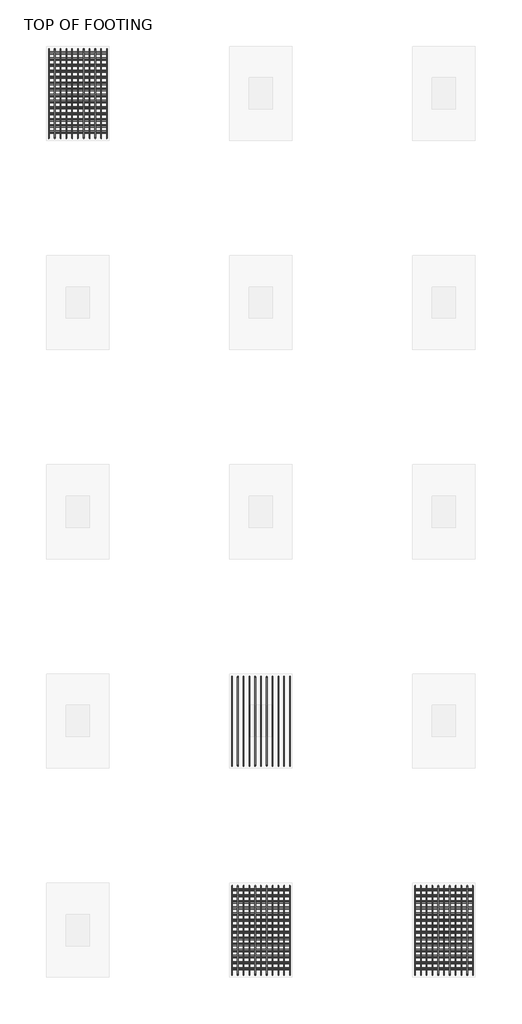
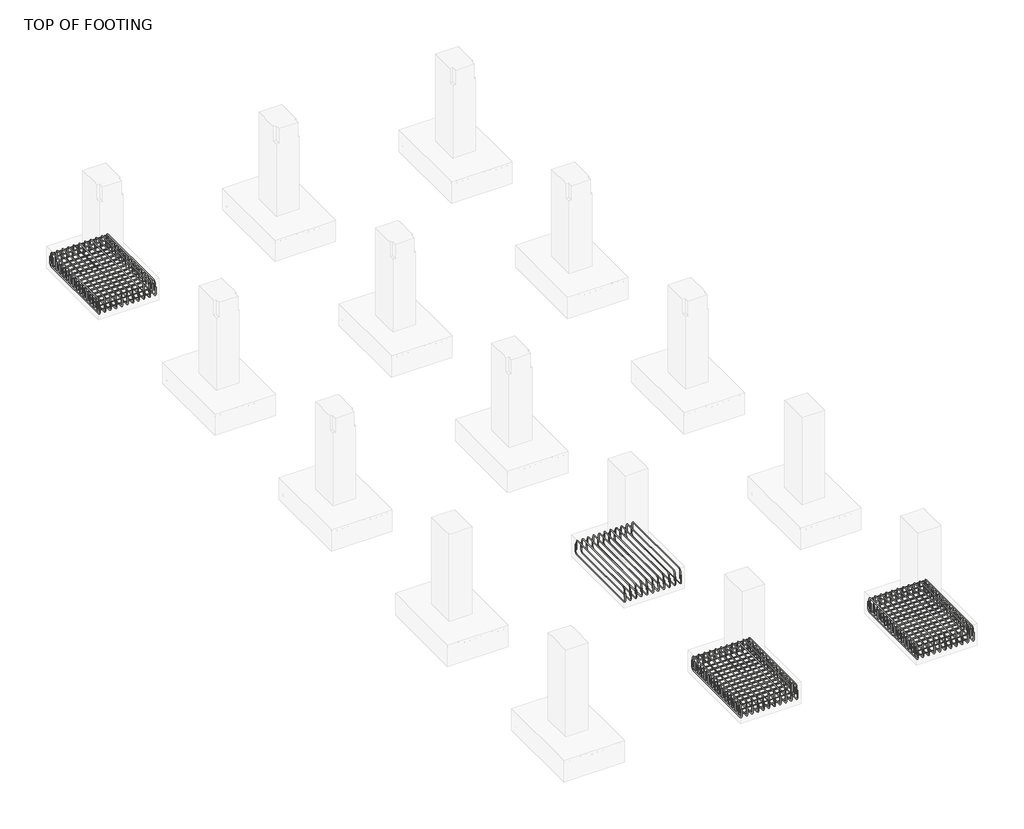
# One storey, part 7 of 11: 14 reinforcing bars.
"""IFC4 building model written with IfcOpenShell, lengths in millimetres."""

from ifc_helpers import new_model, si_unit, point, frame, origin, place, context, project, spatial, polyline, circle_curve, trimmed, segment, composite_curve, source, transform, mapped, element, save
from ifc_brep_helpers import swept_disk

model = new_model("IFC4")

# Units and contexts
model_context = context("Model", 3, world=origin())
ifc_project = project(units=[si_unit("LENGTHUNIT", "METRE", prefix="MILLI")], contexts=[model_context])

# Site, building, storey
site = spatial("IfcSite", under=ifc_project)
building = spatial("IfcBuilding", under=site)
storey = spatial("IfcBuildingStorey", under=building, Name="TOP OF FOOTING", Elevation=-1828.8)

# Reinforcing bars
placement = place(None, origin())
reinforcing_bar_shape = source(origin(), model_context, "Body", "SolidModel", [
    swept_disk(composite_curve([segment(polyline([(-1816.2384094, 18549.4712443, -2012.1658531), (-1816.2384094, 18549.4712443, -2159.4658531)]), True, "CONTINUOUS"), segment(trimmed(circle_curve(frame((-1816.2384094, 18595.8212443, -2159.4658531), z_axis=(1.0, 0.0, 0.0), x_axis=(0.0, -46.35000000000218, 0.0)), 46.35), [point((-1816.2384094, 18549.4712443, -2159.4658531))], [point((-1816.2384094, 18595.8212443, -2205.8158531))], True, "CARTESIAN"), True, "CONTINUOUS"), segment(polyline([(-1816.2384094, 18595.8212443, -2205.8158531), (-1816.2384094, 20210.4212443, -2205.8158531)]), True, "CONTINUOUS"), segment(trimmed(circle_curve(frame((-1816.2384094, 20210.4212443, -2159.4658531), z_axis=(1.0, 0.0, 0.0), x_axis=(0.0, 0.0, -46.34999999999991)), 46.35), [point((-1816.2384094, 20210.4212443, -2205.8158531))], [point((-1816.2384094, 20256.7712443, -2159.4658531))], True, "CARTESIAN"), True, "CONTINUOUS"), segment(polyline([(-1816.2384094, 20256.7712443, -2159.4658531), (-1816.2384094, 20256.7712443, -2012.1658531)]), True, "CONTINUOUS")], self_intersect=False), 6.35),
])
element("IfcReinforcingBar", 1, at=placement, inside=storey, context=model_context, shape_type="MappedRepresentation", body=[
    mapped(reinforcing_bar_shape, transform((0.0, 0.0, 0.0), x_axis=(1.0, 0.0, 0.0), y_axis=(0.0, 1.0, 0.0), z_axis=(0.0, 0.0, 1.0))),
    mapped(reinforcing_bar_shape, transform((-110.73, 0.0, 0.0), x_axis=(1.0, 0.0, 0.0), y_axis=(0.0, 1.0, 0.0), z_axis=(0.0, 0.0, 1.0))),
    mapped(reinforcing_bar_shape, transform((-221.46, 0.0, 0.0), x_axis=(1.0, 0.0, 0.0), y_axis=(0.0, 1.0, 0.0), z_axis=(0.0, 0.0, 1.0))),
    mapped(reinforcing_bar_shape, transform((-332.19, 0.0, 0.0), x_axis=(1.0, 0.0, 0.0), y_axis=(0.0, 1.0, 0.0), z_axis=(0.0, 0.0, 1.0))),
    mapped(reinforcing_bar_shape, transform((-442.92, 0.0, 0.0), x_axis=(1.0, 0.0, 0.0), y_axis=(0.0, 1.0, 0.0), z_axis=(0.0, 0.0, 1.0))),
    mapped(reinforcing_bar_shape, transform((-553.65, 0.0, 0.0), x_axis=(1.0, 0.0, 0.0), y_axis=(0.0, 1.0, 0.0), z_axis=(0.0, 0.0, 1.0))),
    mapped(reinforcing_bar_shape, transform((-664.38, 0.0, 0.0), x_axis=(1.0, 0.0, 0.0), y_axis=(0.0, 1.0, 0.0), z_axis=(0.0, 0.0, 1.0))),
    mapped(reinforcing_bar_shape, transform((-775.11, 0.0, 0.0), x_axis=(1.0, 0.0, 0.0), y_axis=(0.0, 1.0, 0.0), z_axis=(0.0, 0.0, 1.0))),
    mapped(reinforcing_bar_shape, transform((-885.84, 0.0, 0.0), x_axis=(1.0, 0.0, 0.0), y_axis=(0.0, 1.0, 0.0), z_axis=(0.0, 0.0, 1.0))),
    mapped(reinforcing_bar_shape, transform((-996.57, 0.0, 0.0), x_axis=(1.0, 0.0, 0.0), y_axis=(0.0, 1.0, 0.0), z_axis=(0.0, 0.0, 1.0))),
    mapped(reinforcing_bar_shape, transform((-1107.3, 0.0, 0.0), x_axis=(1.0, 0.0, 0.0), y_axis=(0.0, 1.0, 0.0), z_axis=(0.0, 0.0, 1.0))),
])
reinforcing_bar_2_shape = source(origin(), model_context, "Body", "SolidModel", [
    swept_disk(composite_curve([segment(polyline([(-2923.5384094, 18577.6603603, -2096.8914539), (-2923.5384094, 18577.6603603, -1949.5914539)]), True, "CONTINUOUS"), segment(trimmed(circle_curve(frame((-2923.5384094, 18624.0103603, -1949.5914539), z_axis=(-1.0, 0.0, 0.0), x_axis=(0.0, -46.349999999998545, 0.0)), 46.35), [point((-2923.5384094, 18577.6603603, -1949.5914539))], [point((-2923.5384094, 18624.0103603, -1903.2414539))], True, "CARTESIAN"), True, "CONTINUOUS"), segment(polyline([(-2923.5384094, 18624.0103603, -1903.2414539), (-2923.5384094, 20181.3238837, -1903.2414539)]), True, "CONTINUOUS"), segment(trimmed(circle_curve(frame((-2923.5384094, 20181.3238837, -1949.5914539), z_axis=(-1.0, 0.0, 0.0), x_axis=(0.0, 0.0, 46.350000000000136)), 46.35), [point((-2923.5384094, 20181.3238837, -1903.2414539))], [point((-2923.5384094, 20227.6738837, -1949.5914539))], True, "CARTESIAN"), True, "CONTINUOUS"), segment(polyline([(-2923.5384094, 20227.6738837, -1949.5914539), (-2923.5384094, 20227.6738837, -2096.8914539)]), True, "CONTINUOUS")], self_intersect=False), 6.35),
])
element("IfcReinforcingBar", 2, at=placement, inside=storey, context=model_context, shape_type="MappedRepresentation", body=[
    mapped(reinforcing_bar_2_shape, transform((0.0, 0.0, 0.0), x_axis=(1.0, 0.0, 0.0), y_axis=(0.0, 1.0, 0.0), z_axis=(0.0, 0.0, 1.0))),
    mapped(reinforcing_bar_2_shape, transform((110.73, 0.0, 0.0), x_axis=(1.0, 0.0, 0.0), y_axis=(0.0, 1.0, 0.0), z_axis=(0.0, 0.0, 1.0))),
    mapped(reinforcing_bar_2_shape, transform((221.46, 0.0, 0.0), x_axis=(1.0, 0.0, 0.0), y_axis=(0.0, 1.0, 0.0), z_axis=(0.0, 0.0, 1.0))),
    mapped(reinforcing_bar_2_shape, transform((332.19, 0.0, 0.0), x_axis=(1.0, 0.0, 0.0), y_axis=(0.0, 1.0, 0.0), z_axis=(0.0, 0.0, 1.0))),
    mapped(reinforcing_bar_2_shape, transform((442.92, 0.0, 0.0), x_axis=(1.0, 0.0, 0.0), y_axis=(0.0, 1.0, 0.0), z_axis=(0.0, 0.0, 1.0))),
    mapped(reinforcing_bar_2_shape, transform((553.65, 0.0, 0.0), x_axis=(1.0, 0.0, 0.0), y_axis=(0.0, 1.0, 0.0), z_axis=(0.0, 0.0, 1.0))),
    mapped(reinforcing_bar_2_shape, transform((664.38, 0.0, 0.0), x_axis=(1.0, 0.0, 0.0), y_axis=(0.0, 1.0, 0.0), z_axis=(0.0, 0.0, 1.0))),
    mapped(reinforcing_bar_2_shape, transform((775.11, 0.0, 0.0), x_axis=(1.0, 0.0, 0.0), y_axis=(0.0, 1.0, 0.0), z_axis=(0.0, 0.0, 1.0))),
    mapped(reinforcing_bar_2_shape, transform((885.84, 0.0, 0.0), x_axis=(1.0, 0.0, 0.0), y_axis=(0.0, 1.0, 0.0), z_axis=(0.0, 0.0, 1.0))),
    mapped(reinforcing_bar_2_shape, transform((996.57, 0.0, 0.0), x_axis=(1.0, 0.0, 0.0), y_axis=(0.0, 1.0, 0.0), z_axis=(0.0, 0.0, 1.0))),
    mapped(reinforcing_bar_2_shape, transform((1107.3, 0.0, 0.0), x_axis=(1.0, 0.0, 0.0), y_axis=(0.0, 1.0, 0.0), z_axis=(0.0, 0.0, 1.0))),
])
reinforcing_bar_3_shape = source(origin(), model_context, "Body", "SolidModel", [
    swept_disk(composite_curve([segment(polyline([(-2923.5384094, 18653.1930221, -1996.7664426), (-2923.5384094, 18653.1930221, -2144.0664426)]), True, "CONTINUOUS"), segment(trimmed(circle_curve(frame((-2877.1884094, 18653.1930221, -2144.0664426), z_axis=(0.0, -1.0, 0.0), x_axis=(-46.34999999999991, 0.0, 0.0)), 46.35), [point((-2923.5384094, 18653.1930221, -2144.0664426))], [point((-2877.1884094, 18653.1930221, -2190.4164426))], True, "CARTESIAN"), True, "CONTINUOUS"), segment(polyline([(-2877.1884094, 18653.1930221, -2190.4164426), (-1862.5884094, 18653.1930221, -2190.4164426)]), True, "CONTINUOUS"), segment(trimmed(circle_curve(frame((-1862.5884094, 18653.1930221, -2144.0664426), z_axis=(0.0, -1.0, 0.0), x_axis=(0.0, 0.0, -46.350000000000364)), 46.35), [point((-1862.5884094, 18653.1930221, -2190.4164426))], [point((-1816.2384094, 18653.1930221, -2144.0664426))], True, "CARTESIAN"), True, "CONTINUOUS"), segment(polyline([(-1816.2384094, 18653.1930221, -2144.0664426), (-1816.2384094, 18653.1930221, -1996.7664426)]), True, "CONTINUOUS")], self_intersect=False), 6.35),
])
element("IfcReinforcingBar", 3, at=placement, inside=storey, context=model_context, shape_type="MappedRepresentation", body=[
    mapped(reinforcing_bar_3_shape, transform((0.0, 0.0, 0.0), x_axis=(1.0, 0.0, 0.0), y_axis=(0.0, 1.0, 0.0), z_axis=(0.0, 0.0, 1.0))),
    mapped(reinforcing_bar_3_shape, transform((0.0, 116.2744005, 0.0), x_axis=(1.0, 0.0, 0.0), y_axis=(0.0, 1.0, 0.0), z_axis=(0.0, 0.0, 1.0))),
    mapped(reinforcing_bar_3_shape, transform((0.0, 232.5488009, 0.0), x_axis=(1.0, 0.0, 0.0), y_axis=(0.0, 1.0, 0.0), z_axis=(0.0, 0.0, 1.0))),
    mapped(reinforcing_bar_3_shape, transform((0.0, 348.8232014, 0.0), x_axis=(1.0, 0.0, 0.0), y_axis=(0.0, 1.0, 0.0), z_axis=(0.0, 0.0, 1.0))),
    mapped(reinforcing_bar_3_shape, transform((0.0, 465.0976018, 0.0), x_axis=(1.0, 0.0, 0.0), y_axis=(0.0, 1.0, 0.0), z_axis=(0.0, 0.0, 1.0))),
    mapped(reinforcing_bar_3_shape, transform((0.0, 581.3720023, 0.0), x_axis=(1.0, 0.0, 0.0), y_axis=(0.0, 1.0, 0.0), z_axis=(0.0, 0.0, 1.0))),
    mapped(reinforcing_bar_3_shape, transform((0.0, 697.6464027, 0.0), x_axis=(1.0, 0.0, 0.0), y_axis=(0.0, 1.0, 0.0), z_axis=(0.0, 0.0, 1.0))),
    mapped(reinforcing_bar_3_shape, transform((0.0, 813.9208032, 0.0), x_axis=(1.0, 0.0, 0.0), y_axis=(0.0, 1.0, 0.0), z_axis=(0.0, 0.0, 1.0))),
    mapped(reinforcing_bar_3_shape, transform((0.0, 930.1952036, 0.0), x_axis=(1.0, 0.0, 0.0), y_axis=(0.0, 1.0, 0.0), z_axis=(0.0, 0.0, 1.0))),
    mapped(reinforcing_bar_3_shape, transform((0.0, 1046.4696041, 0.0), x_axis=(1.0, 0.0, 0.0), y_axis=(0.0, 1.0, 0.0), z_axis=(0.0, 0.0, 1.0))),
    mapped(reinforcing_bar_3_shape, transform((0.0, 1162.7440045, 0.0), x_axis=(1.0, 0.0, 0.0), y_axis=(0.0, 1.0, 0.0), z_axis=(0.0, 0.0, 1.0))),
    mapped(reinforcing_bar_3_shape, transform((0.0, 1279.018405, 0.0), x_axis=(1.0, 0.0, 0.0), y_axis=(0.0, 1.0, 0.0), z_axis=(0.0, 0.0, 1.0))),
    mapped(reinforcing_bar_3_shape, transform((0.0, 1395.2928054, 0.0), x_axis=(1.0, 0.0, 0.0), y_axis=(0.0, 1.0, 0.0), z_axis=(0.0, 0.0, 1.0))),
    mapped(reinforcing_bar_3_shape, transform((0.0, 1511.5672059, 0.0), x_axis=(1.0, 0.0, 0.0), y_axis=(0.0, 1.0, 0.0), z_axis=(0.0, 0.0, 1.0))),
])
reinforcing_bar_4_shape = source(origin(), model_context, "Body", "SolidModel", [
    swept_disk(composite_curve([segment(polyline([(-2923.5384094, 20194.4257435, -2114.1958609), (-2923.5384094, 20194.4257435, -1966.8958609)]), True, "CONTINUOUS"), segment(trimmed(circle_curve(frame((-2877.1884094, 20194.4257435, -1966.8958609), z_axis=(0.0, 1.0, 0.0), x_axis=(-46.34999999999991, 0.0, 0.0)), 46.35), [point((-2923.5384094, 20194.4257435, -1966.8958609))], [point((-2877.1884094, 20194.4257435, -1920.5458609))], True, "CARTESIAN"), True, "CONTINUOUS"), segment(polyline([(-2877.1884094, 20194.4257435, -1920.5458609), (-1862.5884094, 20194.4257435, -1920.5458609)]), True, "CONTINUOUS"), segment(trimmed(circle_curve(frame((-1862.5884094, 20194.4257435, -1966.8958609), z_axis=(0.0, 1.0, 0.0), x_axis=(0.0, 0.0, 46.34999999999991)), 46.35), [point((-1862.5884094, 20194.4257435, -1920.5458609))], [point((-1816.2384094, 20194.4257435, -1966.8958609))], True, "CARTESIAN"), True, "CONTINUOUS"), segment(polyline([(-1816.2384094, 20194.4257435, -1966.8958609), (-1816.2384094, 20194.4257435, -2114.1958609)]), True, "CONTINUOUS")], self_intersect=False), 6.35),
])
element("IfcReinforcingBar", 4, at=placement, inside=storey, context=model_context, shape_type="MappedRepresentation", body=[
    mapped(reinforcing_bar_4_shape, transform((0.0, 0.0, 0.0), x_axis=(1.0, 0.0, 0.0), y_axis=(0.0, 1.0, 0.0), z_axis=(0.0, 0.0, 1.0))),
    mapped(reinforcing_bar_4_shape, transform((0.0, -116.1057918, 0.0), x_axis=(1.0, 0.0, 0.0), y_axis=(0.0, 1.0, 0.0), z_axis=(0.0, 0.0, 1.0))),
    mapped(reinforcing_bar_4_shape, transform((0.0, -232.2115836, 0.0), x_axis=(1.0, 0.0, 0.0), y_axis=(0.0, 1.0, 0.0), z_axis=(0.0, 0.0, 1.0))),
    mapped(reinforcing_bar_4_shape, transform((0.0, -348.3173754, 0.0), x_axis=(1.0, 0.0, 0.0), y_axis=(0.0, 1.0, 0.0), z_axis=(0.0, 0.0, 1.0))),
    mapped(reinforcing_bar_4_shape, transform((0.0, -464.4231672, 0.0), x_axis=(1.0, 0.0, 0.0), y_axis=(0.0, 1.0, 0.0), z_axis=(0.0, 0.0, 1.0))),
    mapped(reinforcing_bar_4_shape, transform((0.0, -580.528959, 0.0), x_axis=(1.0, 0.0, 0.0), y_axis=(0.0, 1.0, 0.0), z_axis=(0.0, 0.0, 1.0))),
    mapped(reinforcing_bar_4_shape, transform((0.0, -696.6347508, 0.0), x_axis=(1.0, 0.0, 0.0), y_axis=(0.0, 1.0, 0.0), z_axis=(0.0, 0.0, 1.0))),
    mapped(reinforcing_bar_4_shape, transform((0.0, -812.7405426, 0.0), x_axis=(1.0, 0.0, 0.0), y_axis=(0.0, 1.0, 0.0), z_axis=(0.0, 0.0, 1.0))),
    mapped(reinforcing_bar_4_shape, transform((0.0, -928.8463344, 0.0), x_axis=(1.0, 0.0, 0.0), y_axis=(0.0, 1.0, 0.0), z_axis=(0.0, 0.0, 1.0))),
    mapped(reinforcing_bar_4_shape, transform((0.0, -1044.9521262, 0.0), x_axis=(1.0, 0.0, 0.0), y_axis=(0.0, 1.0, 0.0), z_axis=(0.0, 0.0, 1.0))),
    mapped(reinforcing_bar_4_shape, transform((0.0, -1161.057918, 0.0), x_axis=(1.0, 0.0, 0.0), y_axis=(0.0, 1.0, 0.0), z_axis=(0.0, 0.0, 1.0))),
    mapped(reinforcing_bar_4_shape, transform((0.0, -1277.1637098, 0.0), x_axis=(1.0, 0.0, 0.0), y_axis=(0.0, 1.0, 0.0), z_axis=(0.0, 0.0, 1.0))),
    mapped(reinforcing_bar_4_shape, transform((0.0, -1393.2695016, 0.0), x_axis=(1.0, 0.0, 0.0), y_axis=(0.0, 1.0, 0.0), z_axis=(0.0, 0.0, 1.0))),
    mapped(reinforcing_bar_4_shape, transform((0.0, -1509.3752934, 0.0), x_axis=(1.0, 0.0, 0.0), y_axis=(0.0, 1.0, 0.0), z_axis=(0.0, 0.0, 1.0))),
])
reinforcing_bar_5_shape = source(origin(), model_context, "Body", "SolidModel", [
    swept_disk(composite_curve([segment(polyline([(5183.7615906, 2549.4712443, -2012.1658531), (5183.7615906, 2549.4712443, -2159.4658531)]), True, "CONTINUOUS"), segment(trimmed(circle_curve(frame((5183.7615906, 2595.8212443, -2159.4658531), z_axis=(1.0, 0.0, 0.0), x_axis=(0.0, -46.350000000000364, 0.0)), 46.35), [point((5183.7615906, 2549.4712443, -2159.4658531))], [point((5183.7615906, 2595.8212443, -2205.8158531))], True, "CARTESIAN"), True, "CONTINUOUS"), segment(polyline([(5183.7615906, 2595.8212443, -2205.8158531), (5183.7615906, 4210.4212443, -2205.8158531)]), True, "CONTINUOUS"), segment(trimmed(circle_curve(frame((5183.7615906, 4210.4212443, -2159.4658531), z_axis=(1.0, 0.0, 0.0), x_axis=(0.0, 0.0, -46.34999999999991)), 46.35), [point((5183.7615906, 4210.4212443, -2205.8158531))], [point((5183.7615906, 4256.7712443, -2159.4658531))], True, "CARTESIAN"), True, "CONTINUOUS"), segment(polyline([(5183.7615906, 4256.7712443, -2159.4658531), (5183.7615906, 4256.7712443, -2012.1658531)]), True, "CONTINUOUS")], self_intersect=False), 6.35),
])
element("IfcReinforcingBar", 5, at=placement, inside=storey, context=model_context, shape_type="MappedRepresentation", body=[
    mapped(reinforcing_bar_5_shape, transform((0.0, 0.0, 0.0), x_axis=(1.0, 0.0, 0.0), y_axis=(0.0, 1.0, 0.0), z_axis=(0.0, 0.0, 1.0))),
    mapped(reinforcing_bar_5_shape, transform((-110.73, 0.0, 0.0), x_axis=(1.0, 0.0, 0.0), y_axis=(0.0, 1.0, 0.0), z_axis=(0.0, 0.0, 1.0))),
    mapped(reinforcing_bar_5_shape, transform((-221.46, 0.0, 0.0), x_axis=(1.0, 0.0, 0.0), y_axis=(0.0, 1.0, 0.0), z_axis=(0.0, 0.0, 1.0))),
    mapped(reinforcing_bar_5_shape, transform((-332.19, 0.0, 0.0), x_axis=(1.0, 0.0, 0.0), y_axis=(0.0, 1.0, 0.0), z_axis=(0.0, 0.0, 1.0))),
    mapped(reinforcing_bar_5_shape, transform((-442.92, 0.0, 0.0), x_axis=(1.0, 0.0, 0.0), y_axis=(0.0, 1.0, 0.0), z_axis=(0.0, 0.0, 1.0))),
    mapped(reinforcing_bar_5_shape, transform((-553.65, 0.0, 0.0), x_axis=(1.0, 0.0, 0.0), y_axis=(0.0, 1.0, 0.0), z_axis=(0.0, 0.0, 1.0))),
    mapped(reinforcing_bar_5_shape, transform((-664.38, 0.0, 0.0), x_axis=(1.0, 0.0, 0.0), y_axis=(0.0, 1.0, 0.0), z_axis=(0.0, 0.0, 1.0))),
    mapped(reinforcing_bar_5_shape, transform((-775.11, 0.0, 0.0), x_axis=(1.0, 0.0, 0.0), y_axis=(0.0, 1.0, 0.0), z_axis=(0.0, 0.0, 1.0))),
    mapped(reinforcing_bar_5_shape, transform((-885.84, 0.0, 0.0), x_axis=(1.0, 0.0, 0.0), y_axis=(0.0, 1.0, 0.0), z_axis=(0.0, 0.0, 1.0))),
    mapped(reinforcing_bar_5_shape, transform((-996.57, 0.0, 0.0), x_axis=(1.0, 0.0, 0.0), y_axis=(0.0, 1.0, 0.0), z_axis=(0.0, 0.0, 1.0))),
    mapped(reinforcing_bar_5_shape, transform((-1107.3, 0.0, 0.0), x_axis=(1.0, 0.0, 0.0), y_axis=(0.0, 1.0, 0.0), z_axis=(0.0, 0.0, 1.0))),
])
reinforcing_bar_6_shape = source(origin(), model_context, "Body", "SolidModel", [
    swept_disk(composite_curve([segment(polyline([(4076.4615906, 2577.6603603, -2096.8914539), (4076.4615906, 2577.6603603, -1949.5914539)]), True, "CONTINUOUS"), segment(trimmed(circle_curve(frame((4076.4615906, 2624.0103603, -1949.5914539), z_axis=(-1.0, 0.0, 0.0), x_axis=(0.0, -46.34999999999991, 0.0)), 46.35), [point((4076.4615906, 2577.6603603, -1949.5914539))], [point((4076.4615906, 2624.0103603, -1903.2414539))], True, "CARTESIAN"), True, "CONTINUOUS"), segment(polyline([(4076.4615906, 2624.0103603, -1903.2414539), (4076.4615906, 4181.3238837, -1903.2414539)]), True, "CONTINUOUS"), segment(trimmed(circle_curve(frame((4076.4615906, 4181.3238837, -1949.5914539), z_axis=(-1.0, 0.0, 0.0), x_axis=(0.0, 0.0, 46.350000000000136)), 46.35), [point((4076.4615906, 4181.3238837, -1903.2414539))], [point((4076.4615906, 4227.6738837, -1949.5914539))], True, "CARTESIAN"), True, "CONTINUOUS"), segment(polyline([(4076.4615906, 4227.6738837, -1949.5914539), (4076.4615906, 4227.6738837, -2096.8914539)]), True, "CONTINUOUS")], self_intersect=False), 6.35),
])
element("IfcReinforcingBar", 6, at=placement, inside=storey, context=model_context, shape_type="MappedRepresentation", body=[
    mapped(reinforcing_bar_6_shape, transform((0.0, 0.0, 0.0), x_axis=(1.0, 0.0, 0.0), y_axis=(0.0, 1.0, 0.0), z_axis=(0.0, 0.0, 1.0))),
    mapped(reinforcing_bar_6_shape, transform((110.73, 0.0, 0.0), x_axis=(1.0, 0.0, 0.0), y_axis=(0.0, 1.0, 0.0), z_axis=(0.0, 0.0, 1.0))),
    mapped(reinforcing_bar_6_shape, transform((221.46, 0.0, 0.0), x_axis=(1.0, 0.0, 0.0), y_axis=(0.0, 1.0, 0.0), z_axis=(0.0, 0.0, 1.0))),
    mapped(reinforcing_bar_6_shape, transform((332.19, 0.0, 0.0), x_axis=(1.0, 0.0, 0.0), y_axis=(0.0, 1.0, 0.0), z_axis=(0.0, 0.0, 1.0))),
    mapped(reinforcing_bar_6_shape, transform((442.92, 0.0, 0.0), x_axis=(1.0, 0.0, 0.0), y_axis=(0.0, 1.0, 0.0), z_axis=(0.0, 0.0, 1.0))),
    mapped(reinforcing_bar_6_shape, transform((553.65, 0.0, 0.0), x_axis=(1.0, 0.0, 0.0), y_axis=(0.0, 1.0, 0.0), z_axis=(0.0, 0.0, 1.0))),
    mapped(reinforcing_bar_6_shape, transform((664.38, 0.0, 0.0), x_axis=(1.0, 0.0, 0.0), y_axis=(0.0, 1.0, 0.0), z_axis=(0.0, 0.0, 1.0))),
    mapped(reinforcing_bar_6_shape, transform((775.11, 0.0, 0.0), x_axis=(1.0, 0.0, 0.0), y_axis=(0.0, 1.0, 0.0), z_axis=(0.0, 0.0, 1.0))),
    mapped(reinforcing_bar_6_shape, transform((885.84, 0.0, 0.0), x_axis=(1.0, 0.0, 0.0), y_axis=(0.0, 1.0, 0.0), z_axis=(0.0, 0.0, 1.0))),
    mapped(reinforcing_bar_6_shape, transform((996.57, 0.0, 0.0), x_axis=(1.0, 0.0, 0.0), y_axis=(0.0, 1.0, 0.0), z_axis=(0.0, 0.0, 1.0))),
    mapped(reinforcing_bar_6_shape, transform((1107.3, 0.0, 0.0), x_axis=(1.0, 0.0, 0.0), y_axis=(0.0, 1.0, 0.0), z_axis=(0.0, 0.0, 1.0))),
])
reinforcing_bar_7_shape = source(origin(), model_context, "Body", "SolidModel", [
    swept_disk(composite_curve([segment(polyline([(4076.4615906, 2653.1930221, -1996.7664426), (4076.4615906, 2653.1930221, -2144.0664426)]), True, "CONTINUOUS"), segment(trimmed(circle_curve(frame((4122.8115906, 2653.1930221, -2144.0664426), z_axis=(0.0, -1.0, 0.0), x_axis=(-46.350000000000364, 0.0, 0.0)), 46.35), [point((4076.4615906, 2653.1930221, -2144.0664426))], [point((4122.8115906, 2653.1930221, -2190.4164426))], True, "CARTESIAN"), True, "CONTINUOUS"), segment(polyline([(4122.8115906, 2653.1930221, -2190.4164426), (5137.4115906, 2653.1930221, -2190.4164426)]), True, "CONTINUOUS"), segment(trimmed(circle_curve(frame((5137.4115906, 2653.1930221, -2144.0664426), z_axis=(0.0, -1.0, 0.0), x_axis=(0.0, 0.0, -46.350000000000364)), 46.35), [point((5137.4115906, 2653.1930221, -2190.4164426))], [point((5183.7615906, 2653.1930221, -2144.0664426))], True, "CARTESIAN"), True, "CONTINUOUS"), segment(polyline([(5183.7615906, 2653.1930221, -2144.0664426), (5183.7615906, 2653.1930221, -1996.7664426)]), True, "CONTINUOUS")], self_intersect=False), 6.35),
])
element("IfcReinforcingBar", 7, at=placement, inside=storey, context=model_context, shape_type="MappedRepresentation", body=[
    mapped(reinforcing_bar_7_shape, transform((0.0, 0.0, 0.0), x_axis=(1.0, 0.0, 0.0), y_axis=(0.0, 1.0, 0.0), z_axis=(0.0, 0.0, 1.0))),
    mapped(reinforcing_bar_7_shape, transform((0.0, 116.2744005, 0.0), x_axis=(1.0, 0.0, 0.0), y_axis=(0.0, 1.0, 0.0), z_axis=(0.0, 0.0, 1.0))),
    mapped(reinforcing_bar_7_shape, transform((0.0, 232.5488009, 0.0), x_axis=(1.0, 0.0, 0.0), y_axis=(0.0, 1.0, 0.0), z_axis=(0.0, 0.0, 1.0))),
    mapped(reinforcing_bar_7_shape, transform((0.0, 348.8232014, 0.0), x_axis=(1.0, 0.0, 0.0), y_axis=(0.0, 1.0, 0.0), z_axis=(0.0, 0.0, 1.0))),
    mapped(reinforcing_bar_7_shape, transform((0.0, 465.0976018, 0.0), x_axis=(1.0, 0.0, 0.0), y_axis=(0.0, 1.0, 0.0), z_axis=(0.0, 0.0, 1.0))),
    mapped(reinforcing_bar_7_shape, transform((0.0, 581.3720023, 0.0), x_axis=(1.0, 0.0, 0.0), y_axis=(0.0, 1.0, 0.0), z_axis=(0.0, 0.0, 1.0))),
    mapped(reinforcing_bar_7_shape, transform((0.0, 697.6464027, 0.0), x_axis=(1.0, 0.0, 0.0), y_axis=(0.0, 1.0, 0.0), z_axis=(0.0, 0.0, 1.0))),
    mapped(reinforcing_bar_7_shape, transform((0.0, 813.9208032, 0.0), x_axis=(1.0, 0.0, 0.0), y_axis=(0.0, 1.0, 0.0), z_axis=(0.0, 0.0, 1.0))),
    mapped(reinforcing_bar_7_shape, transform((0.0, 930.1952036, 0.0), x_axis=(1.0, 0.0, 0.0), y_axis=(0.0, 1.0, 0.0), z_axis=(0.0, 0.0, 1.0))),
    mapped(reinforcing_bar_7_shape, transform((0.0, 1046.4696041, 0.0), x_axis=(1.0, 0.0, 0.0), y_axis=(0.0, 1.0, 0.0), z_axis=(0.0, 0.0, 1.0))),
    mapped(reinforcing_bar_7_shape, transform((0.0, 1162.7440045, 0.0), x_axis=(1.0, 0.0, 0.0), y_axis=(0.0, 1.0, 0.0), z_axis=(0.0, 0.0, 1.0))),
    mapped(reinforcing_bar_7_shape, transform((0.0, 1279.018405, 0.0), x_axis=(1.0, 0.0, 0.0), y_axis=(0.0, 1.0, 0.0), z_axis=(0.0, 0.0, 1.0))),
    mapped(reinforcing_bar_7_shape, transform((0.0, 1395.2928054, 0.0), x_axis=(1.0, 0.0, 0.0), y_axis=(0.0, 1.0, 0.0), z_axis=(0.0, 0.0, 1.0))),
    mapped(reinforcing_bar_7_shape, transform((0.0, 1511.5672059, 0.0), x_axis=(1.0, 0.0, 0.0), y_axis=(0.0, 1.0, 0.0), z_axis=(0.0, 0.0, 1.0))),
])
reinforcing_bar_8_shape = source(origin(), model_context, "Body", "SolidModel", [
    swept_disk(composite_curve([segment(polyline([(4076.4615906, 4194.4257435, -2114.1958609), (4076.4615906, 4194.4257435, -1966.8958609)]), True, "CONTINUOUS"), segment(trimmed(circle_curve(frame((4122.8115906, 4194.4257435, -1966.8958609), z_axis=(0.0, 1.0, 0.0), x_axis=(-46.350000000000364, 0.0, 0.0)), 46.35), [point((4076.4615906, 4194.4257435, -1966.8958609))], [point((4122.8115906, 4194.4257435, -1920.5458609))], True, "CARTESIAN"), True, "CONTINUOUS"), segment(polyline([(4122.8115906, 4194.4257435, -1920.5458609), (5137.4115906, 4194.4257435, -1920.5458609)]), True, "CONTINUOUS"), segment(trimmed(circle_curve(frame((5137.4115906, 4194.4257435, -1966.8958609), z_axis=(0.0, 1.0, 0.0), x_axis=(0.0, 0.0, 46.34999999999991)), 46.35), [point((5137.4115906, 4194.4257435, -1920.5458609))], [point((5183.7615906, 4194.4257435, -1966.8958609))], True, "CARTESIAN"), True, "CONTINUOUS"), segment(polyline([(5183.7615906, 4194.4257435, -1966.8958609), (5183.7615906, 4194.4257435, -2114.1958609)]), True, "CONTINUOUS")], self_intersect=False), 6.35),
])
element("IfcReinforcingBar", 8, at=placement, inside=storey, context=model_context, shape_type="MappedRepresentation", body=[
    mapped(reinforcing_bar_8_shape, transform((0.0, 0.0, 0.0), x_axis=(1.0, 0.0, 0.0), y_axis=(0.0, 1.0, 0.0), z_axis=(0.0, 0.0, 1.0))),
    mapped(reinforcing_bar_8_shape, transform((0.0, -116.1057918, 0.0), x_axis=(1.0, 0.0, 0.0), y_axis=(0.0, 1.0, 0.0), z_axis=(0.0, 0.0, 1.0))),
    mapped(reinforcing_bar_8_shape, transform((0.0, -232.2115836, 0.0), x_axis=(1.0, 0.0, 0.0), y_axis=(0.0, 1.0, 0.0), z_axis=(0.0, 0.0, 1.0))),
    mapped(reinforcing_bar_8_shape, transform((0.0, -348.3173754, 0.0), x_axis=(1.0, 0.0, 0.0), y_axis=(0.0, 1.0, 0.0), z_axis=(0.0, 0.0, 1.0))),
    mapped(reinforcing_bar_8_shape, transform((0.0, -464.4231672, 0.0), x_axis=(1.0, 0.0, 0.0), y_axis=(0.0, 1.0, 0.0), z_axis=(0.0, 0.0, 1.0))),
    mapped(reinforcing_bar_8_shape, transform((0.0, -580.528959, 0.0), x_axis=(1.0, 0.0, 0.0), y_axis=(0.0, 1.0, 0.0), z_axis=(0.0, 0.0, 1.0))),
    mapped(reinforcing_bar_8_shape, transform((0.0, -696.6347508, 0.0), x_axis=(1.0, 0.0, 0.0), y_axis=(0.0, 1.0, 0.0), z_axis=(0.0, 0.0, 1.0))),
    mapped(reinforcing_bar_8_shape, transform((0.0, -812.7405426, 0.0), x_axis=(1.0, 0.0, 0.0), y_axis=(0.0, 1.0, 0.0), z_axis=(0.0, 0.0, 1.0))),
    mapped(reinforcing_bar_8_shape, transform((0.0, -928.8463344, 0.0), x_axis=(1.0, 0.0, 0.0), y_axis=(0.0, 1.0, 0.0), z_axis=(0.0, 0.0, 1.0))),
    mapped(reinforcing_bar_8_shape, transform((0.0, -1044.9521262, 0.0), x_axis=(1.0, 0.0, 0.0), y_axis=(0.0, 1.0, 0.0), z_axis=(0.0, 0.0, 1.0))),
    mapped(reinforcing_bar_8_shape, transform((0.0, -1161.057918, 0.0), x_axis=(1.0, 0.0, 0.0), y_axis=(0.0, 1.0, 0.0), z_axis=(0.0, 0.0, 1.0))),
    mapped(reinforcing_bar_8_shape, transform((0.0, -1277.1637098, 0.0), x_axis=(1.0, 0.0, 0.0), y_axis=(0.0, 1.0, 0.0), z_axis=(0.0, 0.0, 1.0))),
    mapped(reinforcing_bar_8_shape, transform((0.0, -1393.2695016, 0.0), x_axis=(1.0, 0.0, 0.0), y_axis=(0.0, 1.0, 0.0), z_axis=(0.0, 0.0, 1.0))),
    mapped(reinforcing_bar_8_shape, transform((0.0, -1509.3752934, 0.0), x_axis=(1.0, 0.0, 0.0), y_axis=(0.0, 1.0, 0.0), z_axis=(0.0, 0.0, 1.0))),
])
reinforcing_bar_9_shape = source(origin(), model_context, "Body", "SolidModel", [
    swept_disk(composite_curve([segment(polyline([(1683.7615906, 6549.4712443, -2012.1658531), (1683.7615906, 6549.4712443, -2159.4658531)]), True, "CONTINUOUS"), segment(trimmed(circle_curve(frame((1683.7615906, 6595.8212443, -2159.4658531), z_axis=(1.0, 0.0, 0.0), x_axis=(0.0, -46.350000000000364, 0.0)), 46.35), [point((1683.7615906, 6549.4712443, -2159.4658531))], [point((1683.7615906, 6595.8212443, -2205.8158531))], True, "CARTESIAN"), True, "CONTINUOUS"), segment(polyline([(1683.7615906, 6595.8212443, -2205.8158531), (1683.7615906, 8210.4212443, -2205.8158531)]), True, "CONTINUOUS"), segment(trimmed(circle_curve(frame((1683.7615906, 8210.4212443, -2159.4658531), z_axis=(1.0, 0.0, 0.0), x_axis=(0.0, 0.0, -46.34999999999991)), 46.35), [point((1683.7615906, 8210.4212443, -2205.8158531))], [point((1683.7615906, 8256.7712443, -2159.4658531))], True, "CARTESIAN"), True, "CONTINUOUS"), segment(polyline([(1683.7615906, 8256.7712443, -2159.4658531), (1683.7615906, 8256.7712443, -2012.1658531)]), True, "CONTINUOUS")], self_intersect=False), 6.35),
])
element("IfcReinforcingBar", 9, at=placement, inside=storey, context=model_context, shape_type="MappedRepresentation", body=[
    mapped(reinforcing_bar_9_shape, transform((0.0, 0.0, 0.0), x_axis=(1.0, 0.0, 0.0), y_axis=(0.0, 1.0, 0.0), z_axis=(0.0, 0.0, 1.0))),
    mapped(reinforcing_bar_9_shape, transform((-110.73, 0.0, 0.0), x_axis=(1.0, 0.0, 0.0), y_axis=(0.0, 1.0, 0.0), z_axis=(0.0, 0.0, 1.0))),
    mapped(reinforcing_bar_9_shape, transform((-221.46, 0.0, 0.0), x_axis=(1.0, 0.0, 0.0), y_axis=(0.0, 1.0, 0.0), z_axis=(0.0, 0.0, 1.0))),
    mapped(reinforcing_bar_9_shape, transform((-332.19, 0.0, 0.0), x_axis=(1.0, 0.0, 0.0), y_axis=(0.0, 1.0, 0.0), z_axis=(0.0, 0.0, 1.0))),
    mapped(reinforcing_bar_9_shape, transform((-442.92, 0.0, 0.0), x_axis=(1.0, 0.0, 0.0), y_axis=(0.0, 1.0, 0.0), z_axis=(0.0, 0.0, 1.0))),
    mapped(reinforcing_bar_9_shape, transform((-553.65, 0.0, 0.0), x_axis=(1.0, 0.0, 0.0), y_axis=(0.0, 1.0, 0.0), z_axis=(0.0, 0.0, 1.0))),
    mapped(reinforcing_bar_9_shape, transform((-664.38, 0.0, 0.0), x_axis=(1.0, 0.0, 0.0), y_axis=(0.0, 1.0, 0.0), z_axis=(0.0, 0.0, 1.0))),
    mapped(reinforcing_bar_9_shape, transform((-775.11, 0.0, 0.0), x_axis=(1.0, 0.0, 0.0), y_axis=(0.0, 1.0, 0.0), z_axis=(0.0, 0.0, 1.0))),
    mapped(reinforcing_bar_9_shape, transform((-885.84, 0.0, 0.0), x_axis=(1.0, 0.0, 0.0), y_axis=(0.0, 1.0, 0.0), z_axis=(0.0, 0.0, 1.0))),
    mapped(reinforcing_bar_9_shape, transform((-996.57, 0.0, 0.0), x_axis=(1.0, 0.0, 0.0), y_axis=(0.0, 1.0, 0.0), z_axis=(0.0, 0.0, 1.0))),
    mapped(reinforcing_bar_9_shape, transform((-1107.3, 0.0, 0.0), x_axis=(1.0, 0.0, 0.0), y_axis=(0.0, 1.0, 0.0), z_axis=(0.0, 0.0, 1.0))),
])
reinforcing_bar_10_shape = source(origin(), model_context, "Body", "SolidModel", [
    swept_disk(composite_curve([segment(polyline([(576.4615906, 6577.6603603, -2096.8914539), (576.4615906, 6577.6603603, -1949.5914539)]), True, "CONTINUOUS"), segment(trimmed(circle_curve(frame((576.4615906, 6624.0103603, -1949.5914539), z_axis=(-1.0, 0.0, 0.0), x_axis=(0.0, -46.349999999999454, 0.0)), 46.35), [point((576.4615906, 6577.6603603, -1949.5914539))], [point((576.4615906, 6624.0103603, -1903.2414539))], True, "CARTESIAN"), True, "CONTINUOUS"), segment(polyline([(576.4615906, 6624.0103603, -1903.2414539), (576.4615906, 8181.3238837, -1903.2414539)]), True, "CONTINUOUS"), segment(trimmed(circle_curve(frame((576.4615906, 8181.3238837, -1949.5914539), z_axis=(-1.0, 0.0, 0.0), x_axis=(0.0, 0.0, 46.350000000000136)), 46.35), [point((576.4615906, 8181.3238837, -1903.2414539))], [point((576.4615906, 8227.6738837, -1949.5914539))], True, "CARTESIAN"), True, "CONTINUOUS"), segment(polyline([(576.4615906, 8227.6738837, -1949.5914539), (576.4615906, 8227.6738837, -2096.8914539)]), True, "CONTINUOUS")], self_intersect=False), 6.35),
])
element("IfcReinforcingBar", 10, at=placement, inside=storey, context=model_context, shape_type="MappedRepresentation", body=[
    mapped(reinforcing_bar_10_shape, transform((0.0, 0.0, 0.0), x_axis=(1.0, 0.0, 0.0), y_axis=(0.0, 1.0, 0.0), z_axis=(0.0, 0.0, 1.0))),
    mapped(reinforcing_bar_10_shape, transform((110.73, 0.0, 0.0), x_axis=(1.0, 0.0, 0.0), y_axis=(0.0, 1.0, 0.0), z_axis=(0.0, 0.0, 1.0))),
    mapped(reinforcing_bar_10_shape, transform((221.46, 0.0, 0.0), x_axis=(1.0, 0.0, 0.0), y_axis=(0.0, 1.0, 0.0), z_axis=(0.0, 0.0, 1.0))),
    mapped(reinforcing_bar_10_shape, transform((332.19, 0.0, 0.0), x_axis=(1.0, 0.0, 0.0), y_axis=(0.0, 1.0, 0.0), z_axis=(0.0, 0.0, 1.0))),
    mapped(reinforcing_bar_10_shape, transform((442.92, 0.0, 0.0), x_axis=(1.0, 0.0, 0.0), y_axis=(0.0, 1.0, 0.0), z_axis=(0.0, 0.0, 1.0))),
    mapped(reinforcing_bar_10_shape, transform((553.65, 0.0, 0.0), x_axis=(1.0, 0.0, 0.0), y_axis=(0.0, 1.0, 0.0), z_axis=(0.0, 0.0, 1.0))),
    mapped(reinforcing_bar_10_shape, transform((664.38, 0.0, 0.0), x_axis=(1.0, 0.0, 0.0), y_axis=(0.0, 1.0, 0.0), z_axis=(0.0, 0.0, 1.0))),
    mapped(reinforcing_bar_10_shape, transform((775.11, 0.0, 0.0), x_axis=(1.0, 0.0, 0.0), y_axis=(0.0, 1.0, 0.0), z_axis=(0.0, 0.0, 1.0))),
    mapped(reinforcing_bar_10_shape, transform((885.84, 0.0, 0.0), x_axis=(1.0, 0.0, 0.0), y_axis=(0.0, 1.0, 0.0), z_axis=(0.0, 0.0, 1.0))),
    mapped(reinforcing_bar_10_shape, transform((996.57, 0.0, 0.0), x_axis=(1.0, 0.0, 0.0), y_axis=(0.0, 1.0, 0.0), z_axis=(0.0, 0.0, 1.0))),
    mapped(reinforcing_bar_10_shape, transform((1107.3, 0.0, 0.0), x_axis=(1.0, 0.0, 0.0), y_axis=(0.0, 1.0, 0.0), z_axis=(0.0, 0.0, 1.0))),
])
reinforcing_bar_11_shape = source(origin(), model_context, "Body", "SolidModel", [
    swept_disk(composite_curve([segment(polyline([(1683.7615906, 2549.4712443, -2012.1658531), (1683.7615906, 2549.4712443, -2159.4658531)]), True, "CONTINUOUS"), segment(trimmed(circle_curve(frame((1683.7615906, 2595.8212443, -2159.4658531), z_axis=(1.0, 0.0, 0.0), x_axis=(0.0, -46.350000000000364, 0.0)), 46.35), [point((1683.7615906, 2549.4712443, -2159.4658531))], [point((1683.7615906, 2595.8212443, -2205.8158531))], True, "CARTESIAN"), True, "CONTINUOUS"), segment(polyline([(1683.7615906, 2595.8212443, -2205.8158531), (1683.7615906, 4210.4212443, -2205.8158531)]), True, "CONTINUOUS"), segment(trimmed(circle_curve(frame((1683.7615906, 4210.4212443, -2159.4658531), z_axis=(1.0, 0.0, 0.0), x_axis=(0.0, 0.0, -46.34999999999991)), 46.35), [point((1683.7615906, 4210.4212443, -2205.8158531))], [point((1683.7615906, 4256.7712443, -2159.4658531))], True, "CARTESIAN"), True, "CONTINUOUS"), segment(polyline([(1683.7615906, 4256.7712443, -2159.4658531), (1683.7615906, 4256.7712443, -2012.1658531)]), True, "CONTINUOUS")], self_intersect=False), 6.35),
])
element("IfcReinforcingBar", 11, at=placement, inside=storey, context=model_context, shape_type="MappedRepresentation", body=[
    mapped(reinforcing_bar_11_shape, transform((0.0, 0.0, 0.0), x_axis=(1.0, 0.0, 0.0), y_axis=(0.0, 1.0, 0.0), z_axis=(0.0, 0.0, 1.0))),
    mapped(reinforcing_bar_11_shape, transform((-110.73, 0.0, 0.0), x_axis=(1.0, 0.0, 0.0), y_axis=(0.0, 1.0, 0.0), z_axis=(0.0, 0.0, 1.0))),
    mapped(reinforcing_bar_11_shape, transform((-221.46, 0.0, 0.0), x_axis=(1.0, 0.0, 0.0), y_axis=(0.0, 1.0, 0.0), z_axis=(0.0, 0.0, 1.0))),
    mapped(reinforcing_bar_11_shape, transform((-332.19, 0.0, 0.0), x_axis=(1.0, 0.0, 0.0), y_axis=(0.0, 1.0, 0.0), z_axis=(0.0, 0.0, 1.0))),
    mapped(reinforcing_bar_11_shape, transform((-442.92, 0.0, 0.0), x_axis=(1.0, 0.0, 0.0), y_axis=(0.0, 1.0, 0.0), z_axis=(0.0, 0.0, 1.0))),
    mapped(reinforcing_bar_11_shape, transform((-553.65, 0.0, 0.0), x_axis=(1.0, 0.0, 0.0), y_axis=(0.0, 1.0, 0.0), z_axis=(0.0, 0.0, 1.0))),
    mapped(reinforcing_bar_11_shape, transform((-664.38, 0.0, 0.0), x_axis=(1.0, 0.0, 0.0), y_axis=(0.0, 1.0, 0.0), z_axis=(0.0, 0.0, 1.0))),
    mapped(reinforcing_bar_11_shape, transform((-775.11, 0.0, 0.0), x_axis=(1.0, 0.0, 0.0), y_axis=(0.0, 1.0, 0.0), z_axis=(0.0, 0.0, 1.0))),
    mapped(reinforcing_bar_11_shape, transform((-885.84, 0.0, 0.0), x_axis=(1.0, 0.0, 0.0), y_axis=(0.0, 1.0, 0.0), z_axis=(0.0, 0.0, 1.0))),
    mapped(reinforcing_bar_11_shape, transform((-996.57, 0.0, 0.0), x_axis=(1.0, 0.0, 0.0), y_axis=(0.0, 1.0, 0.0), z_axis=(0.0, 0.0, 1.0))),
    mapped(reinforcing_bar_11_shape, transform((-1107.3, 0.0, 0.0), x_axis=(1.0, 0.0, 0.0), y_axis=(0.0, 1.0, 0.0), z_axis=(0.0, 0.0, 1.0))),
])
reinforcing_bar_12_shape = source(origin(), model_context, "Body", "SolidModel", [
    swept_disk(composite_curve([segment(polyline([(576.4615906, 2577.6603603, -2096.8914539), (576.4615906, 2577.6603603, -1949.5914539)]), True, "CONTINUOUS"), segment(trimmed(circle_curve(frame((576.4615906, 2624.0103603, -1949.5914539), z_axis=(-1.0, 0.0, 0.0), x_axis=(0.0, -46.34999999999991, 0.0)), 46.35), [point((576.4615906, 2577.6603603, -1949.5914539))], [point((576.4615906, 2624.0103603, -1903.2414539))], True, "CARTESIAN"), True, "CONTINUOUS"), segment(polyline([(576.4615906, 2624.0103603, -1903.2414539), (576.4615906, 4181.3238837, -1903.2414539)]), True, "CONTINUOUS"), segment(trimmed(circle_curve(frame((576.4615906, 4181.3238837, -1949.5914539), z_axis=(-1.0, 0.0, 0.0), x_axis=(0.0, 0.0, 46.350000000000136)), 46.35), [point((576.4615906, 4181.3238837, -1903.2414539))], [point((576.4615906, 4227.6738837, -1949.5914539))], True, "CARTESIAN"), True, "CONTINUOUS"), segment(polyline([(576.4615906, 4227.6738837, -1949.5914539), (576.4615906, 4227.6738837, -2096.8914539)]), True, "CONTINUOUS")], self_intersect=False), 6.35),
])
element("IfcReinforcingBar", 12, at=placement, inside=storey, context=model_context, shape_type="MappedRepresentation", body=[
    mapped(reinforcing_bar_12_shape, transform((0.0, 0.0, 0.0), x_axis=(1.0, 0.0, 0.0), y_axis=(0.0, 1.0, 0.0), z_axis=(0.0, 0.0, 1.0))),
    mapped(reinforcing_bar_12_shape, transform((110.73, 0.0, 0.0), x_axis=(1.0, 0.0, 0.0), y_axis=(0.0, 1.0, 0.0), z_axis=(0.0, 0.0, 1.0))),
    mapped(reinforcing_bar_12_shape, transform((221.46, 0.0, 0.0), x_axis=(1.0, 0.0, 0.0), y_axis=(0.0, 1.0, 0.0), z_axis=(0.0, 0.0, 1.0))),
    mapped(reinforcing_bar_12_shape, transform((332.19, 0.0, 0.0), x_axis=(1.0, 0.0, 0.0), y_axis=(0.0, 1.0, 0.0), z_axis=(0.0, 0.0, 1.0))),
    mapped(reinforcing_bar_12_shape, transform((442.92, 0.0, 0.0), x_axis=(1.0, 0.0, 0.0), y_axis=(0.0, 1.0, 0.0), z_axis=(0.0, 0.0, 1.0))),
    mapped(reinforcing_bar_12_shape, transform((553.65, 0.0, 0.0), x_axis=(1.0, 0.0, 0.0), y_axis=(0.0, 1.0, 0.0), z_axis=(0.0, 0.0, 1.0))),
    mapped(reinforcing_bar_12_shape, transform((664.38, 0.0, 0.0), x_axis=(1.0, 0.0, 0.0), y_axis=(0.0, 1.0, 0.0), z_axis=(0.0, 0.0, 1.0))),
    mapped(reinforcing_bar_12_shape, transform((775.11, 0.0, 0.0), x_axis=(1.0, 0.0, 0.0), y_axis=(0.0, 1.0, 0.0), z_axis=(0.0, 0.0, 1.0))),
    mapped(reinforcing_bar_12_shape, transform((885.84, 0.0, 0.0), x_axis=(1.0, 0.0, 0.0), y_axis=(0.0, 1.0, 0.0), z_axis=(0.0, 0.0, 1.0))),
    mapped(reinforcing_bar_12_shape, transform((996.57, 0.0, 0.0), x_axis=(1.0, 0.0, 0.0), y_axis=(0.0, 1.0, 0.0), z_axis=(0.0, 0.0, 1.0))),
    mapped(reinforcing_bar_12_shape, transform((1107.3, 0.0, 0.0), x_axis=(1.0, 0.0, 0.0), y_axis=(0.0, 1.0, 0.0), z_axis=(0.0, 0.0, 1.0))),
])
reinforcing_bar_13_shape = source(origin(), model_context, "Body", "SolidModel", [
    swept_disk(composite_curve([segment(polyline([(576.4615906, 2653.1930221, -1996.7664426), (576.4615906, 2653.1930221, -2144.0664426)]), True, "CONTINUOUS"), segment(trimmed(circle_curve(frame((622.8115906, 2653.1930221, -2144.0664426), z_axis=(0.0, -1.0, 0.0), x_axis=(-46.35000000000002, 0.0, 0.0)), 46.35), [point((576.4615906, 2653.1930221, -2144.0664426))], [point((622.8115906, 2653.1930221, -2190.4164426))], True, "CARTESIAN"), True, "CONTINUOUS"), segment(polyline([(622.8115906, 2653.1930221, -2190.4164426), (1637.4115906, 2653.1930221, -2190.4164426)]), True, "CONTINUOUS"), segment(trimmed(circle_curve(frame((1637.4115906, 2653.1930221, -2144.0664426), z_axis=(0.0, -1.0, 0.0), x_axis=(0.0, 0.0, -46.350000000000364)), 46.35), [point((1637.4115906, 2653.1930221, -2190.4164426))], [point((1683.7615906, 2653.1930221, -2144.0664426))], True, "CARTESIAN"), True, "CONTINUOUS"), segment(polyline([(1683.7615906, 2653.1930221, -2144.0664426), (1683.7615906, 2653.1930221, -1996.7664426)]), True, "CONTINUOUS")], self_intersect=False), 6.35),
])
element("IfcReinforcingBar", 13, at=placement, inside=storey, context=model_context, shape_type="MappedRepresentation", body=[
    mapped(reinforcing_bar_13_shape, transform((0.0, 0.0, 0.0), x_axis=(1.0, 0.0, 0.0), y_axis=(0.0, 1.0, 0.0), z_axis=(0.0, 0.0, 1.0))),
    mapped(reinforcing_bar_13_shape, transform((0.0, 116.2744005, 0.0), x_axis=(1.0, 0.0, 0.0), y_axis=(0.0, 1.0, 0.0), z_axis=(0.0, 0.0, 1.0))),
    mapped(reinforcing_bar_13_shape, transform((0.0, 232.5488009, 0.0), x_axis=(1.0, 0.0, 0.0), y_axis=(0.0, 1.0, 0.0), z_axis=(0.0, 0.0, 1.0))),
    mapped(reinforcing_bar_13_shape, transform((0.0, 348.8232014, 0.0), x_axis=(1.0, 0.0, 0.0), y_axis=(0.0, 1.0, 0.0), z_axis=(0.0, 0.0, 1.0))),
    mapped(reinforcing_bar_13_shape, transform((0.0, 465.0976018, 0.0), x_axis=(1.0, 0.0, 0.0), y_axis=(0.0, 1.0, 0.0), z_axis=(0.0, 0.0, 1.0))),
    mapped(reinforcing_bar_13_shape, transform((0.0, 581.3720023, 0.0), x_axis=(1.0, 0.0, 0.0), y_axis=(0.0, 1.0, 0.0), z_axis=(0.0, 0.0, 1.0))),
    mapped(reinforcing_bar_13_shape, transform((0.0, 697.6464027, 0.0), x_axis=(1.0, 0.0, 0.0), y_axis=(0.0, 1.0, 0.0), z_axis=(0.0, 0.0, 1.0))),
    mapped(reinforcing_bar_13_shape, transform((0.0, 813.9208032, 0.0), x_axis=(1.0, 0.0, 0.0), y_axis=(0.0, 1.0, 0.0), z_axis=(0.0, 0.0, 1.0))),
    mapped(reinforcing_bar_13_shape, transform((0.0, 930.1952036, 0.0), x_axis=(1.0, 0.0, 0.0), y_axis=(0.0, 1.0, 0.0), z_axis=(0.0, 0.0, 1.0))),
    mapped(reinforcing_bar_13_shape, transform((0.0, 1046.4696041, 0.0), x_axis=(1.0, 0.0, 0.0), y_axis=(0.0, 1.0, 0.0), z_axis=(0.0, 0.0, 1.0))),
    mapped(reinforcing_bar_13_shape, transform((0.0, 1162.7440045, 0.0), x_axis=(1.0, 0.0, 0.0), y_axis=(0.0, 1.0, 0.0), z_axis=(0.0, 0.0, 1.0))),
    mapped(reinforcing_bar_13_shape, transform((0.0, 1279.018405, 0.0), x_axis=(1.0, 0.0, 0.0), y_axis=(0.0, 1.0, 0.0), z_axis=(0.0, 0.0, 1.0))),
    mapped(reinforcing_bar_13_shape, transform((0.0, 1395.2928054, 0.0), x_axis=(1.0, 0.0, 0.0), y_axis=(0.0, 1.0, 0.0), z_axis=(0.0, 0.0, 1.0))),
    mapped(reinforcing_bar_13_shape, transform((0.0, 1511.5672059, 0.0), x_axis=(1.0, 0.0, 0.0), y_axis=(0.0, 1.0, 0.0), z_axis=(0.0, 0.0, 1.0))),
])
reinforcing_bar_14_shape = source(origin(), model_context, "Body", "SolidModel", [
    swept_disk(composite_curve([segment(polyline([(576.4615906, 4194.4257435, -2114.1958609), (576.4615906, 4194.4257435, -1966.8958609)]), True, "CONTINUOUS"), segment(trimmed(circle_curve(frame((622.8115906, 4194.4257435, -1966.8958609), z_axis=(0.0, 1.0, 0.0), x_axis=(-46.35000000000002, 0.0, 0.0)), 46.35), [point((576.4615906, 4194.4257435, -1966.8958609))], [point((622.8115906, 4194.4257435, -1920.5458609))], True, "CARTESIAN"), True, "CONTINUOUS"), segment(polyline([(622.8115906, 4194.4257435, -1920.5458609), (1637.4115906, 4194.4257435, -1920.5458609)]), True, "CONTINUOUS"), segment(trimmed(circle_curve(frame((1637.4115906, 4194.4257435, -1966.8958609), z_axis=(0.0, 1.0, 0.0), x_axis=(0.0, 0.0, 46.34999999999991)), 46.35), [point((1637.4115906, 4194.4257435, -1920.5458609))], [point((1683.7615906, 4194.4257435, -1966.8958609))], True, "CARTESIAN"), True, "CONTINUOUS"), segment(polyline([(1683.7615906, 4194.4257435, -1966.8958609), (1683.7615906, 4194.4257435, -2114.1958609)]), True, "CONTINUOUS")], self_intersect=False), 6.35),
])
element("IfcReinforcingBar", 14, at=placement, inside=storey, context=model_context, shape_type="MappedRepresentation", body=[
    mapped(reinforcing_bar_14_shape, transform((0.0, 0.0, 0.0), x_axis=(1.0, 0.0, 0.0), y_axis=(0.0, 1.0, 0.0), z_axis=(0.0, 0.0, 1.0))),
    mapped(reinforcing_bar_14_shape, transform((0.0, -116.1057918, 0.0), x_axis=(1.0, 0.0, 0.0), y_axis=(0.0, 1.0, 0.0), z_axis=(0.0, 0.0, 1.0))),
    mapped(reinforcing_bar_14_shape, transform((0.0, -232.2115836, 0.0), x_axis=(1.0, 0.0, 0.0), y_axis=(0.0, 1.0, 0.0), z_axis=(0.0, 0.0, 1.0))),
    mapped(reinforcing_bar_14_shape, transform((0.0, -348.3173754, 0.0), x_axis=(1.0, 0.0, 0.0), y_axis=(0.0, 1.0, 0.0), z_axis=(0.0, 0.0, 1.0))),
    mapped(reinforcing_bar_14_shape, transform((0.0, -464.4231672, 0.0), x_axis=(1.0, 0.0, 0.0), y_axis=(0.0, 1.0, 0.0), z_axis=(0.0, 0.0, 1.0))),
    mapped(reinforcing_bar_14_shape, transform((0.0, -580.528959, 0.0), x_axis=(1.0, 0.0, 0.0), y_axis=(0.0, 1.0, 0.0), z_axis=(0.0, 0.0, 1.0))),
    mapped(reinforcing_bar_14_shape, transform((0.0, -696.6347508, 0.0), x_axis=(1.0, 0.0, 0.0), y_axis=(0.0, 1.0, 0.0), z_axis=(0.0, 0.0, 1.0))),
    mapped(reinforcing_bar_14_shape, transform((0.0, -812.7405426, 0.0), x_axis=(1.0, 0.0, 0.0), y_axis=(0.0, 1.0, 0.0), z_axis=(0.0, 0.0, 1.0))),
    mapped(reinforcing_bar_14_shape, transform((0.0, -928.8463344, 0.0), x_axis=(1.0, 0.0, 0.0), y_axis=(0.0, 1.0, 0.0), z_axis=(0.0, 0.0, 1.0))),
    mapped(reinforcing_bar_14_shape, transform((0.0, -1044.9521262, 0.0), x_axis=(1.0, 0.0, 0.0), y_axis=(0.0, 1.0, 0.0), z_axis=(0.0, 0.0, 1.0))),
    mapped(reinforcing_bar_14_shape, transform((0.0, -1161.057918, 0.0), x_axis=(1.0, 0.0, 0.0), y_axis=(0.0, 1.0, 0.0), z_axis=(0.0, 0.0, 1.0))),
    mapped(reinforcing_bar_14_shape, transform((0.0, -1277.1637098, 0.0), x_axis=(1.0, 0.0, 0.0), y_axis=(0.0, 1.0, 0.0), z_axis=(0.0, 0.0, 1.0))),
    mapped(reinforcing_bar_14_shape, transform((0.0, -1393.2695016, 0.0), x_axis=(1.0, 0.0, 0.0), y_axis=(0.0, 1.0, 0.0), z_axis=(0.0, 0.0, 1.0))),
    mapped(reinforcing_bar_14_shape, transform((0.0, -1509.3752934, 0.0), x_axis=(1.0, 0.0, 0.0), y_axis=(0.0, 1.0, 0.0), z_axis=(0.0, 0.0, 1.0))),
])

save(model, "model.ifc")

# Revit data of these elements
# Elements 1, 2, 3, 4, 5, 6, 7, 8, 9, 10, 11, 12, 13, 14 (IfcReinforcingBar)
#   Phase Created = New Construction
